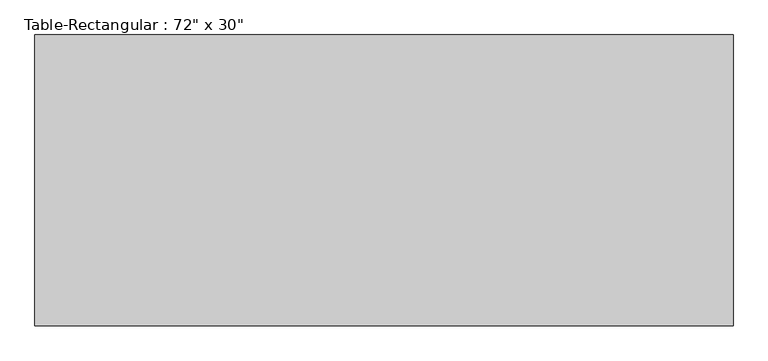
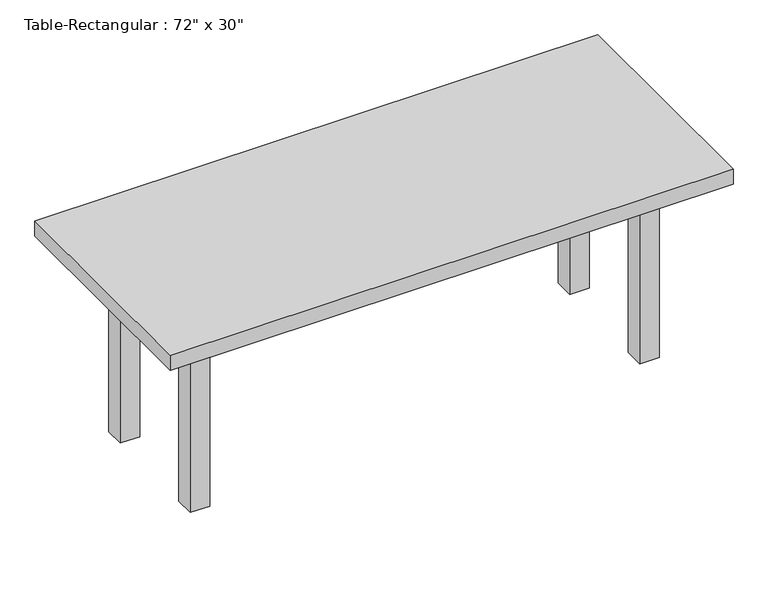
"""IFC4 building model written with IfcOpenShell, lengths in millimetres: furniture geometry."""

from ifc_helpers import new_model, si_unit, frame, origin, origin_with_axes, place, context, project, spatial, polyline, outline, extrude, source, transform, mapped, element, save


def furniture_62ce4b1f(model_context):
    return source(origin(), model_context, "Body", "SweptSolid", [
        extrude(outline(polyline([(698.5, 190.5), (698.5, 165.1), (-698.5, 165.1), (-698.5, 190.5), (698.5, 190.5)])), frame((0.0, 0.0, 533.4), z_axis=(0.0, 0.0, 1.0), x_axis=(1.0, 0.0, 0.0)), (0.0, 0.0, 1.0), 101.6),
        extrude(outline(polyline([(698.5, -190.5), (-698.5, -190.5), (-698.5, -165.1), (698.5, -165.1), (698.5, -190.5)])), frame((0.0, 0.0, 533.4), z_axis=(0.0, 0.0, 1.0), x_axis=(1.0, 0.0, 0.0)), (0.0, 0.0, 1.0), 101.6),
        extrude(outline(polyline([(-711.2, -165.1), (-736.6, -165.1), (-736.6, 165.1), (-711.2, 165.1), (-711.2, -165.1)])), frame((0.0, 0.0, 533.4), z_axis=(0.0, 0.0, 1.0), x_axis=(1.0, 0.0, 0.0)), (0.0, 0.0, 1.0), 101.6),
        extrude(outline(polyline([(711.2, -165.1), (711.2, 165.1), (736.6, 165.1), (736.6, -165.1), (711.2, -165.1)])), frame((0.0, 0.0, 533.4), z_axis=(0.0, 0.0, 1.0), x_axis=(1.0, 0.0, 0.0)), (0.0, 0.0, 1.0), 101.6),
        extrude(outline(polyline([(914.4, 381.0), (914.4, -381.0), (-914.4, -381.0), (-914.4, 381.0), (914.4, 381.0)])), frame((0.0, 0.0, 635.0), z_axis=(0.0, 0.0, 1.0), x_axis=(1.0, 0.0, 0.0)), (0.0, 0.0, 1.0), 50.8),
        extrude(outline(polyline([(-698.5, 228.6), (-698.5, 165.1), (-762.0, 165.1), (-762.0, 228.6), (-698.5, 228.6)])), origin_with_axes(), (0.0, 0.0, 1.0), 635.0),
        extrude(outline(polyline([(698.5, 228.6), (762.0, 228.6), (762.0, 165.1), (698.5, 165.1), (698.5, 228.6)])), origin_with_axes(), (0.0, 0.0, 1.0), 635.0),
        extrude(outline(polyline([(-698.5, -228.6), (-762.0, -228.6), (-762.0, -165.1), (-698.5, -165.1), (-698.5, -228.6)])), origin_with_axes(), (0.0, 0.0, 1.0), 635.0),
        extrude(outline(polyline([(698.5, -228.6), (698.5, -165.1), (762.0, -165.1), (762.0, -228.6), (698.5, -228.6)])), origin_with_axes(), (0.0, 0.0, 1.0), 635.0),
    ])


if __name__ == "__main__":
    model = new_model("IFC4")
    model_context = context("Model", 3, world=origin())
    ifc_project = project(units=[si_unit("LENGTHUNIT", "METRE", prefix="MILLI")], contexts=[model_context])
    site = spatial("IfcSite", under=ifc_project)
    building = spatial("IfcBuilding", under=site)
    placement = place(None, origin())
    furniture_shape = furniture_62ce4b1f(model_context)
    element("IfcFurniture", 1, ObjectType="Table-Rectangular : 72\" x 30\"", at=placement, inside=building, context=model_context, shape_type="MappedRepresentation", body=[
        mapped(furniture_shape, transform((0.0, 0.0, 0.0), x_axis=(1.0, 0.0, 0.0), y_axis=(0.0, 1.0, 0.0), z_axis=(0.0, 0.0, 1.0))),
    ])
    save(model, "model.ifc")

# Revit data of these elements
# Type "Table-Rectangular : 72\" x 30\""
#   Assembly Code = "E2020200"
#   Height = 2' - 3"
#   Length = 6' - 0"
#   Width = 2' - 6"
#   Base Material = Birch
#   Top Material = Birch
#   Default Elevation = 0
# Element 1 (IfcFurniture, "Table-Rectangular : 72\" x 30\"")
#   Materials on its faces: "Birch"
# Materials
#   "Birch": class "Wood", colour RGB 224 178 126, transparency 0, Description = "Betula Alleghaniensis", Cost = 0
